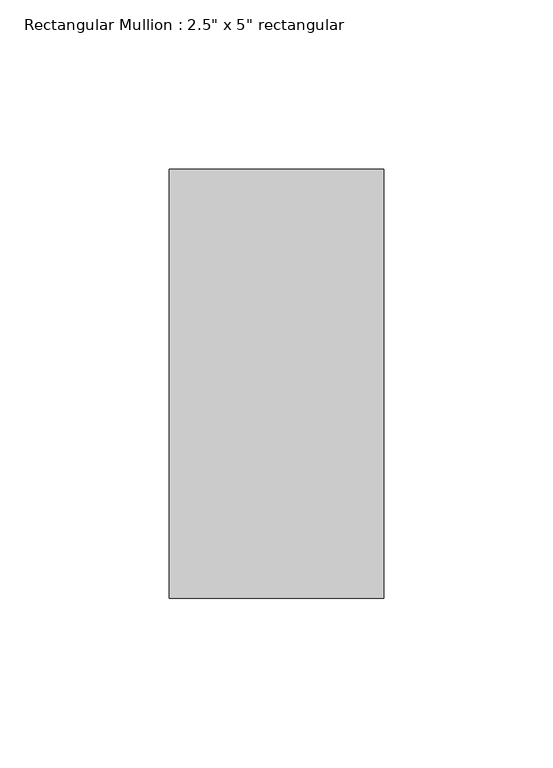
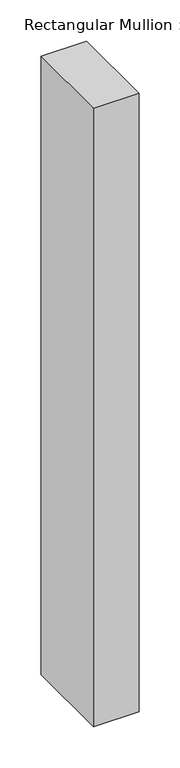
"""IFC4 building model written with IfcOpenShell, lengths in millimetres: member geometry."""

from ifc_helpers import new_model, si_unit, frame, origin, place, context, project, spatial, polyline, outline, extrude, source, transform, mapped, element, save


def member_73c23c35(model_context):
    return source(origin(), model_context, "Body", "SweptSolid", [
        extrude(outline(polyline([(0.0, 63.5), (0.0, -63.5), (-63.5, -63.5), (-63.5, 63.5), (0.0, 63.5)])), frame((0.0, 0.0, -914.4), z_axis=(0.0, 0.0, 1.0), x_axis=(1.0, 0.0, 0.0)), (0.0, 0.0, 1.0), 914.4),
    ])


if __name__ == "__main__":
    model = new_model("IFC4")
    model_context = context("Model", 3, world=origin())
    ifc_project = project(units=[si_unit("LENGTHUNIT", "METRE", prefix="MILLI")], contexts=[model_context])
    site = spatial("IfcSite", under=ifc_project)
    building = spatial("IfcBuilding", under=site)
    placement = place(None, origin())
    member_shape = member_73c23c35(model_context)
    element("IfcMember", 1, ObjectType="Rectangular Mullion : 2.5\" x 5\" rectangular", at=placement, inside=building, context=model_context, shape_type="MappedRepresentation", body=[
        mapped(member_shape, transform((0.0, 0.0, 0.0), x_axis=(1.0, 0.0, 0.0), y_axis=(0.0, 1.0, 0.0), z_axis=(0.0, 0.0, 1.0))),
    ])
    save(model, "model.ifc")

# Revit data of these elements
# Type "Rectangular Mullion : 2.5\" x 5\" rectangular"
#   built-in parameter 1007304 = 0.416667 (stored number, unit not read)
#   built-in parameter 1007301 = 0.104167 (stored number, unit not read)
#   built-in parameter 1007300 = 0.104167 (stored number, unit not read)
# Element 1 (IfcMember, "Rectangular Mullion : 2.5\" x 5\" rectangular")
#   Materials on its faces: "WINDOW FRAMING"
# Materials
#   "WINDOW FRAMING": class "Generic", colour RGB 120 120 120, transparency 0, Cost = 0
